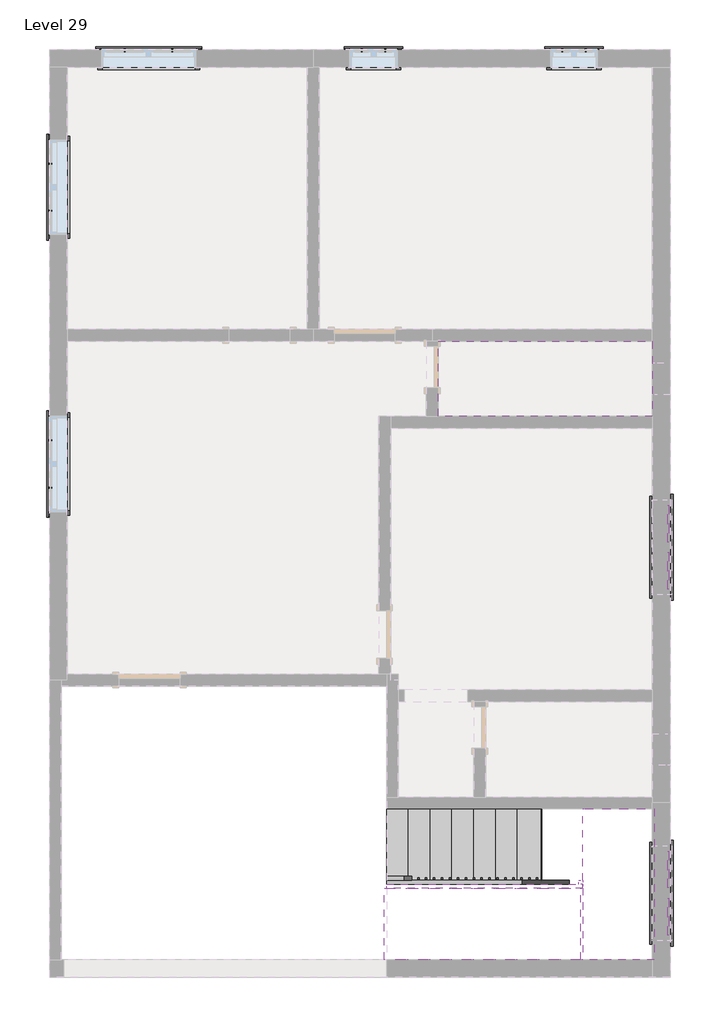
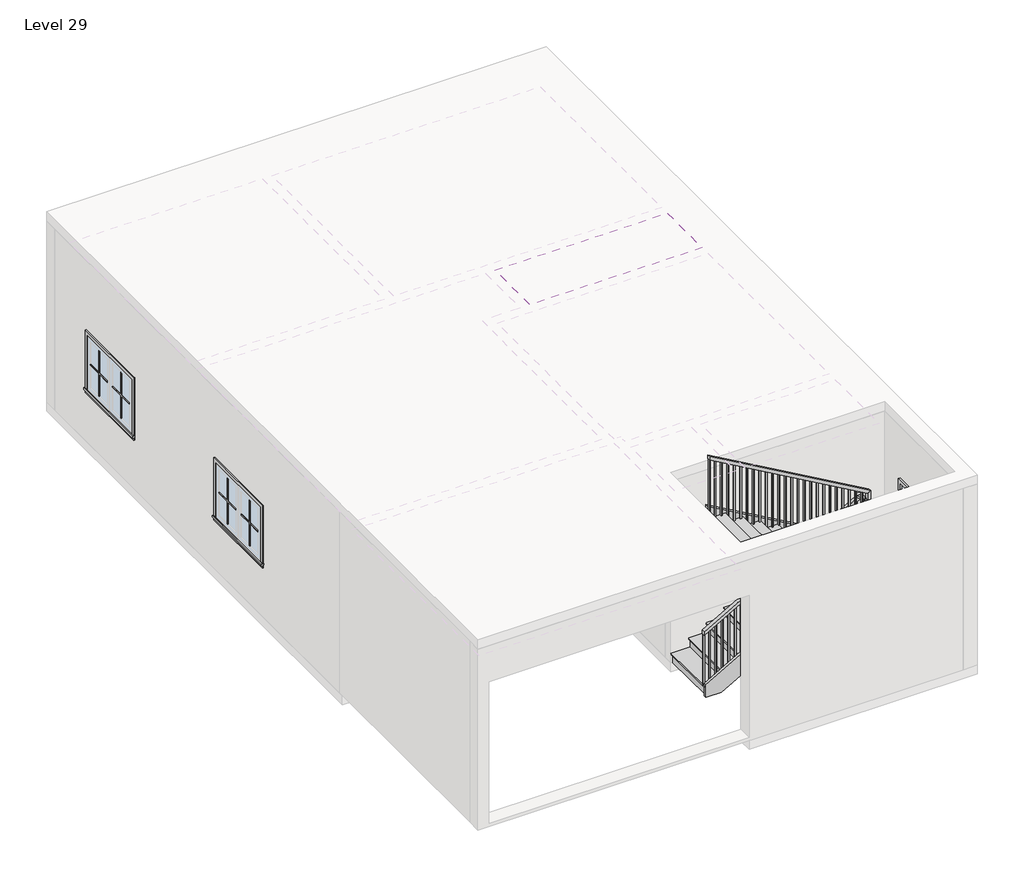
# One storey, part 2 of 2: 44 proxies, 3 members, 2 stair flights, 1 covering, 1 railing, 1 slab.
"""IFC4 building model written with IfcOpenShell, lengths in millimetres."""

from ifc_helpers import new_model, si_unit, frame, origin, place, context, project, spatial, polyline, outline, extrude, faceted_brep, transform, mapped, element, save
from components import muntin_pattern_2x2_muntin_pattern_2x2_2357e71d, muntin_pattern_2x2_muntin_pattern_2x2_302d8f29, muntin_pattern_2x2_muntin_pattern_2x2_53152e2c, muntin_pattern_2x2_muntin_pattern_2x2_e8f3e573, trim_window_exterior_flat_with_sill_c4e67c73, trim_window_exterior_flat_with_sill_a665a915, trim_window_interior_flat_picture_frame_cf1733af, trim_window_interior_flat_picture_frame_d485c387, non_monolithic_landing_9a06da9a, stair_flight_ff2ce9cd, stair_flight_de0ef723

model = new_model("IFC4")

# Units and contexts
model_context = context("Model", 3, world=origin())
ifc_project = project(units=[si_unit("LENGTHUNIT", "METRE", prefix="MILLI")], contexts=[model_context])

# Site, building, storey
site = spatial("IfcSite", under=ifc_project)
building = spatial("IfcBuilding", under=site)
storey = spatial("IfcBuildingStorey", under=building, Name="Level 29", Elevation=25603.2)

# Proxies
placement = place(None, origin())
muntin_pattern_2x2_muntin_pattern_2x2_shape = muntin_pattern_2x2_muntin_pattern_2x2_2357e71d(model_context)
element("IfcBuildingElementProxy", 1, Name="Muntin Pattern_2x2 : Muntin Pattern_2x2", ObjectType="Muntin Pattern_2x2 : Muntin Pattern_2x2", at=placement, inside=storey, context=model_context, shape_type="MappedRepresentation", body=[
    mapped(muntin_pattern_2x2_muntin_pattern_2x2_shape, transform((-4942.3279463, 5897.3080275, 26587.45), x_axis=(1.0, 0.0, 0.0), y_axis=(0.0, 1.0, 0.0), z_axis=(0.0, 0.0, 1.0))),
])
element("IfcBuildingElementProxy", 2, Name="Muntin Pattern_2x2 : Muntin Pattern_2x2", ObjectType="Muntin Pattern_2x2 : Muntin Pattern_2x2", at=placement, inside=storey, context=model_context, shape_type="MappedRepresentation", body=[
    mapped(muntin_pattern_2x2_muntin_pattern_2x2_shape, transform((-5899.5904463, 3838.3205275, 26587.45), x_axis=(0.0, 1.0, 0.0), y_axis=(-1.0, 0.0, 0.0), z_axis=(0.0, 0.0, 1.0))),
])
element("IfcBuildingElementProxy", 3, Name="Muntin Pattern_2x2 : Muntin Pattern_2x2", ObjectType="Muntin Pattern_2x2 : Muntin Pattern_2x2", at=placement, inside=storey, context=model_context, shape_type="MappedRepresentation", body=[
    mapped(muntin_pattern_2x2_muntin_pattern_2x2_shape, transform((-5899.5904463, 293.4330275, 26587.45), x_axis=(0.0, 1.0, 0.0), y_axis=(-1.0, 0.0, 0.0), z_axis=(0.0, 0.0, 1.0))),
])
element("IfcBuildingElementProxy", 4, Name="Muntin Pattern_2x2 : Muntin Pattern_2x2", ObjectType="Muntin Pattern_2x2 : Muntin Pattern_2x2", at=placement, inside=storey, context=model_context, shape_type="MappedRepresentation", body=[
    mapped(muntin_pattern_2x2_muntin_pattern_2x2_shape, transform((2031.5595537, -166.9419725, 26892.25), x_axis=(0.0, -1.0, 0.0), y_axis=(1.0, 0.0, 0.0), z_axis=(0.0, 0.0, 1.0))),
])
element("IfcBuildingElementProxy", 5, Name="Muntin Pattern_2x2 : Muntin Pattern_2x2", ObjectType="Muntin Pattern_2x2 : Muntin Pattern_2x2", at=placement, inside=storey, context=model_context, shape_type="MappedRepresentation", body=[
    mapped(muntin_pattern_2x2_muntin_pattern_2x2_shape, transform((2031.5595537, -4599.2419725, 26892.25), x_axis=(0.0, -1.0, 0.0), y_axis=(1.0, 0.0, 0.0), z_axis=(0.0, 0.0, 1.0))),
])
element("IfcBuildingElementProxy", 6, Name="Muntin Pattern_2x2 : Muntin Pattern_2x2", ObjectType="Muntin Pattern_2x2 : Muntin Pattern_2x2", at=placement, inside=storey, context=model_context, shape_type="MappedRepresentation", body=[
    mapped(muntin_pattern_2x2_muntin_pattern_2x2_shape, transform((-4942.3279463, 5897.3080275, 26587.45), x_axis=(1.0, 0.0, 0.0), y_axis=(0.0, 1.0, 0.0), z_axis=(0.0, 0.0, 1.0))),
])
element("IfcBuildingElementProxy", 7, Name="Muntin Pattern_2x2 : Muntin Pattern_2x2", ObjectType="Muntin Pattern_2x2 : Muntin Pattern_2x2", at=placement, inside=storey, context=model_context, shape_type="MappedRepresentation", body=[
    mapped(muntin_pattern_2x2_muntin_pattern_2x2_shape, transform((2031.5595537, -4599.2419725, 26892.25), x_axis=(0.0, -1.0, 0.0), y_axis=(1.0, 0.0, 0.0), z_axis=(0.0, 0.0, 1.0))),
])
muntin_pattern_2x2_muntin_pattern_2x2_2_shape = muntin_pattern_2x2_muntin_pattern_2x2_302d8f29(model_context)
element("IfcBuildingElementProxy", 8, Name="Muntin Pattern_2x2 : Muntin Pattern_2x2", ObjectType="Muntin Pattern_2x2 : Muntin Pattern_2x2", at=placement, inside=storey, context=model_context, shape_type="MappedRepresentation", body=[
    mapped(muntin_pattern_2x2_muntin_pattern_2x2_2_shape, transform((-4335.9029463, 5897.3080275, 26587.45), x_axis=(-1.0, 0.0, 0.0), y_axis=(0.0, -1.0, 0.0), z_axis=(0.0, 0.0, 1.0))),
])
element("IfcBuildingElementProxy", 9, Name="Muntin Pattern_2x2 : Muntin Pattern_2x2", ObjectType="Muntin Pattern_2x2 : Muntin Pattern_2x2", at=placement, inside=storey, context=model_context, shape_type="MappedRepresentation", body=[
    mapped(muntin_pattern_2x2_muntin_pattern_2x2_2_shape, transform((-5899.5904463, 4444.7455275, 26587.45), x_axis=(0.0, -1.0, 0.0), y_axis=(1.0, 0.0, 0.0), z_axis=(0.0, 0.0, 1.0))),
])
element("IfcBuildingElementProxy", 10, Name="Muntin Pattern_2x2 : Muntin Pattern_2x2", ObjectType="Muntin Pattern_2x2 : Muntin Pattern_2x2", at=placement, inside=storey, context=model_context, shape_type="MappedRepresentation", body=[
    mapped(muntin_pattern_2x2_muntin_pattern_2x2_2_shape, transform((-5899.5904463, 899.8580275, 26587.45), x_axis=(0.0, -1.0, 0.0), y_axis=(1.0, 0.0, 0.0), z_axis=(0.0, 0.0, 1.0))),
])
element("IfcBuildingElementProxy", 11, Name="Muntin Pattern_2x2 : Muntin Pattern_2x2", ObjectType="Muntin Pattern_2x2 : Muntin Pattern_2x2", at=placement, inside=storey, context=model_context, shape_type="MappedRepresentation", body=[
    mapped(muntin_pattern_2x2_muntin_pattern_2x2_2_shape, transform((2031.5595537, -773.3669725, 26892.25), x_axis=(0.0, 1.0, 0.0), y_axis=(-1.0, 0.0, 0.0), z_axis=(0.0, 0.0, 1.0))),
])
element("IfcBuildingElementProxy", 12, Name="Muntin Pattern_2x2 : Muntin Pattern_2x2", ObjectType="Muntin Pattern_2x2 : Muntin Pattern_2x2", at=placement, inside=storey, context=model_context, shape_type="MappedRepresentation", body=[
    mapped(muntin_pattern_2x2_muntin_pattern_2x2_2_shape, transform((2031.5595537, -5205.6669725, 26892.25), x_axis=(0.0, 1.0, 0.0), y_axis=(-1.0, 0.0, 0.0), z_axis=(0.0, 0.0, 1.0))),
])
element("IfcBuildingElementProxy", 13, Name="Muntin Pattern_2x2 : Muntin Pattern_2x2", ObjectType="Muntin Pattern_2x2 : Muntin Pattern_2x2", at=placement, inside=storey, context=model_context, shape_type="MappedRepresentation", body=[
    mapped(muntin_pattern_2x2_muntin_pattern_2x2_2_shape, transform((-4335.9029463, 5897.3080275, 26587.45), x_axis=(-1.0, 0.0, 0.0), y_axis=(0.0, -1.0, 0.0), z_axis=(0.0, 0.0, 1.0))),
])
element("IfcBuildingElementProxy", 14, Name="Muntin Pattern_2x2 : Muntin Pattern_2x2", ObjectType="Muntin Pattern_2x2 : Muntin Pattern_2x2", at=placement, inside=storey, context=model_context, shape_type="MappedRepresentation", body=[
    mapped(muntin_pattern_2x2_muntin_pattern_2x2_2_shape, transform((2031.5595537, -5205.6669725, 26892.25), x_axis=(0.0, 1.0, 0.0), y_axis=(-1.0, 0.0, 0.0), z_axis=(0.0, 0.0, 1.0))),
])
muntin_pattern_2x2_muntin_pattern_2x2_3_shape = muntin_pattern_2x2_muntin_pattern_2x2_53152e2c(model_context)
element("IfcBuildingElementProxy", 15, Name="Muntin Pattern_2x2 : Muntin Pattern_2x2", ObjectType="Muntin Pattern_2x2 : Muntin Pattern_2x2", at=placement, inside=storey, context=model_context, shape_type="MappedRepresentation", body=[
    mapped(muntin_pattern_2x2_muntin_pattern_2x2_3_shape, transform((-1907.0279463, 5897.3080275, 26587.45), x_axis=(1.0, 0.0, 0.0), y_axis=(0.0, 1.0, 0.0), z_axis=(0.0, 0.0, 1.0))),
])
element("IfcBuildingElementProxy", 16, Name="Muntin Pattern_2x2 : Muntin Pattern_2x2", ObjectType="Muntin Pattern_2x2 : Muntin Pattern_2x2", at=placement, inside=storey, context=model_context, shape_type="MappedRepresentation", body=[
    mapped(muntin_pattern_2x2_muntin_pattern_2x2_3_shape, transform((658.3720537, 5897.3080275, 26587.45), x_axis=(1.0, 0.0, 0.0), y_axis=(0.0, 1.0, 0.0), z_axis=(0.0, 0.0, 1.0))),
])
element("IfcBuildingElementProxy", 17, Name="Muntin Pattern_2x2 : Muntin Pattern_2x2", ObjectType="Muntin Pattern_2x2 : Muntin Pattern_2x2", at=placement, inside=storey, context=model_context, shape_type="MappedRepresentation", body=[
    mapped(muntin_pattern_2x2_muntin_pattern_2x2_3_shape, transform((-1907.0279463, 5897.3080275, 26587.45), x_axis=(1.0, 0.0, 0.0), y_axis=(0.0, 1.0, 0.0), z_axis=(0.0, 0.0, 1.0))),
])
element("IfcBuildingElementProxy", 18, Name="Muntin Pattern_2x2 : Muntin Pattern_2x2", ObjectType="Muntin Pattern_2x2 : Muntin Pattern_2x2", at=placement, inside=storey, context=model_context, shape_type="MappedRepresentation", body=[
    mapped(muntin_pattern_2x2_muntin_pattern_2x2_3_shape, transform((658.3720537, 5897.3080275, 26587.45), x_axis=(1.0, 0.0, 0.0), y_axis=(0.0, 1.0, 0.0), z_axis=(0.0, 0.0, 1.0))),
])
muntin_pattern_2x2_muntin_pattern_2x2_4_shape = muntin_pattern_2x2_muntin_pattern_2x2_e8f3e573(model_context)
element("IfcBuildingElementProxy", 19, Name="Muntin Pattern_2x2 : Muntin Pattern_2x2", ObjectType="Muntin Pattern_2x2 : Muntin Pattern_2x2", at=placement, inside=storey, context=model_context, shape_type="MappedRepresentation", body=[
    mapped(muntin_pattern_2x2_muntin_pattern_2x2_4_shape, transform((-1605.4029463, 5897.3080275, 26587.45), x_axis=(-1.0, 0.0, 0.0), y_axis=(0.0, -1.0, 0.0), z_axis=(0.0, 0.0, 1.0))),
])
element("IfcBuildingElementProxy", 20, Name="Muntin Pattern_2x2 : Muntin Pattern_2x2", ObjectType="Muntin Pattern_2x2 : Muntin Pattern_2x2", at=placement, inside=storey, context=model_context, shape_type="MappedRepresentation", body=[
    mapped(muntin_pattern_2x2_muntin_pattern_2x2_4_shape, transform((959.9970537, 5897.3080275, 26587.45), x_axis=(-1.0, 0.0, 0.0), y_axis=(0.0, -1.0, 0.0), z_axis=(0.0, 0.0, 1.0))),
])
element("IfcBuildingElementProxy", 21, Name="Muntin Pattern_2x2 : Muntin Pattern_2x2", ObjectType="Muntin Pattern_2x2 : Muntin Pattern_2x2", at=placement, inside=storey, context=model_context, shape_type="MappedRepresentation", body=[
    mapped(muntin_pattern_2x2_muntin_pattern_2x2_4_shape, transform((-1605.4029463, 5897.3080275, 26587.45), x_axis=(-1.0, 0.0, 0.0), y_axis=(0.0, -1.0, 0.0), z_axis=(0.0, 0.0, 1.0))),
])
element("IfcBuildingElementProxy", 22, Name="Muntin Pattern_2x2 : Muntin Pattern_2x2", ObjectType="Muntin Pattern_2x2 : Muntin Pattern_2x2", at=placement, inside=storey, context=model_context, shape_type="MappedRepresentation", body=[
    mapped(muntin_pattern_2x2_muntin_pattern_2x2_4_shape, transform((959.9970537, 5897.3080275, 26587.45), x_axis=(-1.0, 0.0, 0.0), y_axis=(0.0, -1.0, 0.0), z_axis=(0.0, 0.0, 1.0))),
])
trim_window_exterior_flat_with_sill_shape = trim_window_exterior_flat_with_sill_c4e67c73(model_context)
element("IfcBuildingElementProxy", 23, Name="Trim-Window-Exterior-Flat : with Sill", ObjectType="Trim-Window-Exterior-Flat : with Sill", at=placement, inside=storey, context=model_context, shape_type="MappedRepresentation", body=[
    mapped(trim_window_exterior_flat_with_sill_shape, transform((-4639.1154463, 5906.8330275, 27432.0), x_axis=(-1.0, 0.0, 0.0), y_axis=(0.0, 0.0, 1.0), z_axis=(0.0, 1.0, 0.0))),
])
element("IfcBuildingElementProxy", 24, Name="Trim-Window-Exterior-Flat : with Sill", ObjectType="Trim-Window-Exterior-Flat : with Sill", at=placement, inside=storey, context=model_context, shape_type="MappedRepresentation", body=[
    mapped(trim_window_exterior_flat_with_sill_shape, transform((-5909.1154463, 4141.5330275, 27432.0), x_axis=(0.0, -1.0, 0.0), y_axis=(0.0, 0.0, 1.0), z_axis=(-1.0, 0.0, 0.0))),
])
element("IfcBuildingElementProxy", 25, Name="Trim-Window-Exterior-Flat : with Sill", ObjectType="Trim-Window-Exterior-Flat : with Sill", at=placement, inside=storey, context=model_context, shape_type="MappedRepresentation", body=[
    mapped(trim_window_exterior_flat_with_sill_shape, transform((-5909.1154463, 596.6455275, 27432.0), x_axis=(0.0, -1.0, 0.0), y_axis=(0.0, 0.0, 1.0), z_axis=(-1.0, 0.0, 0.0))),
])
element("IfcBuildingElementProxy", 26, Name="Trim-Window-Exterior-Flat : with Sill", ObjectType="Trim-Window-Exterior-Flat : with Sill", at=placement, inside=storey, context=model_context, shape_type="MappedRepresentation", body=[
    mapped(trim_window_exterior_flat_with_sill_shape, transform((2041.0845537, -470.1544725, 27736.8), x_axis=(0.0, 1.0, 0.0), y_axis=(0.0, 0.0, 1.0), z_axis=(1.0, 0.0, 0.0))),
])
element("IfcBuildingElementProxy", 27, Name="Trim-Window-Exterior-Flat : with Sill", ObjectType="Trim-Window-Exterior-Flat : with Sill", at=placement, inside=storey, context=model_context, shape_type="MappedRepresentation", body=[
    mapped(trim_window_exterior_flat_with_sill_shape, transform((2041.0845537, -4902.4544725, 27736.8), x_axis=(0.0, 1.0, 0.0), y_axis=(0.0, 0.0, 1.0), z_axis=(1.0, 0.0, 0.0))),
])
element("IfcBuildingElementProxy", 28, Name="Trim-Window-Exterior-Flat : with Sill", ObjectType="Trim-Window-Exterior-Flat : with Sill", at=placement, inside=storey, context=model_context, shape_type="MappedRepresentation", body=[
    mapped(trim_window_exterior_flat_with_sill_shape, transform((-4639.1154463, 5906.8330275, 27432.0), x_axis=(-1.0, 0.0, 0.0), y_axis=(0.0, 0.0, 1.0), z_axis=(0.0, 1.0, 0.0))),
])
element("IfcBuildingElementProxy", 29, Name="Trim-Window-Exterior-Flat : with Sill", ObjectType="Trim-Window-Exterior-Flat : with Sill", at=placement, inside=storey, context=model_context, shape_type="MappedRepresentation", body=[
    mapped(trim_window_exterior_flat_with_sill_shape, transform((2041.0845537, -4902.4544725, 27736.8), x_axis=(0.0, 1.0, 0.0), y_axis=(0.0, 0.0, 1.0), z_axis=(1.0, 0.0, 0.0))),
])
trim_window_exterior_flat_with_sill_2_shape = trim_window_exterior_flat_with_sill_a665a915(model_context)
element("IfcBuildingElementProxy", 30, Name="Trim-Window-Exterior-Flat : with Sill", ObjectType="Trim-Window-Exterior-Flat : with Sill", at=placement, inside=storey, context=model_context, shape_type="MappedRepresentation", body=[
    mapped(trim_window_exterior_flat_with_sill_2_shape, transform((-1756.2154463, 5906.8330275, 27432.0), x_axis=(-1.0, 0.0, 0.0), y_axis=(0.0, 0.0, 1.0), z_axis=(0.0, 1.0, 0.0))),
])
element("IfcBuildingElementProxy", 31, Name="Trim-Window-Exterior-Flat : with Sill", ObjectType="Trim-Window-Exterior-Flat : with Sill", at=placement, inside=storey, context=model_context, shape_type="MappedRepresentation", body=[
    mapped(trim_window_exterior_flat_with_sill_2_shape, transform((809.1845537, 5906.8330275, 27432.0), x_axis=(-1.0, 0.0, 0.0), y_axis=(0.0, 0.0, 1.0), z_axis=(0.0, 1.0, 0.0))),
])
element("IfcBuildingElementProxy", 32, Name="Trim-Window-Exterior-Flat : with Sill", ObjectType="Trim-Window-Exterior-Flat : with Sill", at=placement, inside=storey, context=model_context, shape_type="MappedRepresentation", body=[
    mapped(trim_window_exterior_flat_with_sill_2_shape, transform((-1756.2154463, 5906.8330275, 27432.0), x_axis=(-1.0, 0.0, 0.0), y_axis=(0.0, 0.0, 1.0), z_axis=(0.0, 1.0, 0.0))),
])
element("IfcBuildingElementProxy", 33, Name="Trim-Window-Exterior-Flat : with Sill", ObjectType="Trim-Window-Exterior-Flat : with Sill", at=placement, inside=storey, context=model_context, shape_type="MappedRepresentation", body=[
    mapped(trim_window_exterior_flat_with_sill_2_shape, transform((809.1845537, 5906.8330275, 27432.0), x_axis=(-1.0, 0.0, 0.0), y_axis=(0.0, 0.0, 1.0), z_axis=(0.0, 1.0, 0.0))),
])
trim_window_interior_flat_picture_frame_shape = trim_window_interior_flat_picture_frame_cf1733af(model_context)
element("IfcBuildingElementProxy", 34, Name="Trim-Window-Interior-Flat : Picture Frame", ObjectType="Trim-Window-Interior-Flat : Picture Frame", at=placement, inside=storey, context=model_context, shape_type="MappedRepresentation", body=[
    mapped(trim_window_interior_flat_picture_frame_shape, transform((-4639.1154463, 5678.2330275, 27432.0), x_axis=(1.0, 0.0, 0.0), y_axis=(0.0, 0.0, 1.0), z_axis=(0.0, -1.0, 0.0))),
])
element("IfcBuildingElementProxy", 35, Name="Trim-Window-Interior-Flat : Picture Frame", ObjectType="Trim-Window-Interior-Flat : Picture Frame", at=placement, inside=storey, context=model_context, shape_type="MappedRepresentation", body=[
    mapped(trim_window_interior_flat_picture_frame_shape, transform((-5680.5154463, 4141.5330275, 27432.0), x_axis=(0.0, 1.0, 0.0), y_axis=(0.0, 0.0, 1.0), z_axis=(1.0, 0.0, 0.0))),
])
element("IfcBuildingElementProxy", 36, Name="Trim-Window-Interior-Flat : Picture Frame", ObjectType="Trim-Window-Interior-Flat : Picture Frame", at=placement, inside=storey, context=model_context, shape_type="MappedRepresentation", body=[
    mapped(trim_window_interior_flat_picture_frame_shape, transform((-5680.5154463, 596.6455275, 27432.0), x_axis=(0.0, 1.0, 0.0), y_axis=(0.0, 0.0, 1.0), z_axis=(1.0, 0.0, 0.0))),
])
element("IfcBuildingElementProxy", 37, Name="Trim-Window-Interior-Flat : Picture Frame", ObjectType="Trim-Window-Interior-Flat : Picture Frame", at=placement, inside=storey, context=model_context, shape_type="MappedRepresentation", body=[
    mapped(trim_window_interior_flat_picture_frame_shape, transform((1812.4845537, -470.1544725, 27736.8), x_axis=(0.0, -1.0, 0.0), y_axis=(0.0, 0.0, 1.0), z_axis=(-1.0, 0.0, 0.0))),
])
element("IfcBuildingElementProxy", 38, Name="Trim-Window-Interior-Flat : Picture Frame", ObjectType="Trim-Window-Interior-Flat : Picture Frame", at=placement, inside=storey, context=model_context, shape_type="MappedRepresentation", body=[
    mapped(trim_window_interior_flat_picture_frame_shape, transform((1812.4845537, -4902.4544725, 27736.8), x_axis=(0.0, -1.0, 0.0), y_axis=(0.0, 0.0, 1.0), z_axis=(-1.0, 0.0, 0.0))),
])
element("IfcBuildingElementProxy", 39, Name="Trim-Window-Interior-Flat : Picture Frame", ObjectType="Trim-Window-Interior-Flat : Picture Frame", at=placement, inside=storey, context=model_context, shape_type="MappedRepresentation", body=[
    mapped(trim_window_interior_flat_picture_frame_shape, transform((-4639.1154463, 5678.2330275, 27432.0), x_axis=(1.0, 0.0, 0.0), y_axis=(0.0, 0.0, 1.0), z_axis=(0.0, -1.0, 0.0))),
])
element("IfcBuildingElementProxy", 40, Name="Trim-Window-Interior-Flat : Picture Frame", ObjectType="Trim-Window-Interior-Flat : Picture Frame", at=placement, inside=storey, context=model_context, shape_type="MappedRepresentation", body=[
    mapped(trim_window_interior_flat_picture_frame_shape, transform((1812.4845537, -4902.4544725, 27736.8), x_axis=(0.0, -1.0, 0.0), y_axis=(0.0, 0.0, 1.0), z_axis=(-1.0, 0.0, 0.0))),
])
trim_window_interior_flat_picture_frame_2_shape = trim_window_interior_flat_picture_frame_d485c387(model_context)
element("IfcBuildingElementProxy", 41, Name="Trim-Window-Interior-Flat : Picture Frame", ObjectType="Trim-Window-Interior-Flat : Picture Frame", at=placement, inside=storey, context=model_context, shape_type="MappedRepresentation", body=[
    mapped(trim_window_interior_flat_picture_frame_2_shape, transform((-1756.2154463, 5678.2330275, 27432.0), x_axis=(1.0, 0.0, 0.0), y_axis=(0.0, 0.0, 1.0), z_axis=(0.0, -1.0, 0.0))),
])
element("IfcBuildingElementProxy", 42, Name="Trim-Window-Interior-Flat : Picture Frame", ObjectType="Trim-Window-Interior-Flat : Picture Frame", at=placement, inside=storey, context=model_context, shape_type="MappedRepresentation", body=[
    mapped(trim_window_interior_flat_picture_frame_2_shape, transform((809.1845537, 5678.2330275, 27432.0), x_axis=(1.0, 0.0, 0.0), y_axis=(0.0, 0.0, 1.0), z_axis=(0.0, -1.0, 0.0))),
])
element("IfcBuildingElementProxy", 43, Name="Trim-Window-Interior-Flat : Picture Frame", ObjectType="Trim-Window-Interior-Flat : Picture Frame", at=placement, inside=storey, context=model_context, shape_type="MappedRepresentation", body=[
    mapped(trim_window_interior_flat_picture_frame_2_shape, transform((-1756.2154463, 5678.2330275, 27432.0), x_axis=(1.0, 0.0, 0.0), y_axis=(0.0, 0.0, 1.0), z_axis=(0.0, -1.0, 0.0))),
])
element("IfcBuildingElementProxy", 44, Name="Trim-Window-Interior-Flat : Picture Frame", ObjectType="Trim-Window-Interior-Flat : Picture Frame", at=placement, inside=storey, context=model_context, shape_type="MappedRepresentation", body=[
    mapped(trim_window_interior_flat_picture_frame_2_shape, transform((809.1845537, 5678.2330275, 27432.0), x_axis=(1.0, 0.0, 0.0), y_axis=(0.0, 0.0, 1.0), z_axis=(0.0, -1.0, 0.0))),
])

# Covering
element("IfcCovering", 45, ObjectType="2' x 4' ACT System", at=placement, inside=storey, context=model_context, shape_type="SweptSolid", body=[
    extrude(outline(polyline([(-930.7154463, 2171.4455275), (1812.4845537, 2171.4455275), (1812.4845537, 1206.2455275), (-930.7154463, 1206.2455275), (-930.7154463, 2171.4455275)])), frame((0.0, 0.0, 28346.4), z_axis=(0.0, 0.0, 1.0), x_axis=(1.0, 0.0, 0.0)), (0.0, 0.0, 1.0), 57.15),
])

# Members
element("IfcMember", 46, ObjectType="Stringer - 2\" Width", at=placement, inside=storey, context=model_context, shape_type="SweptSolid", body=[
    extrude(outline(polyline([(25812.2890626, -1591.1154463), (25603.2, -1591.1154463), (25603.2, -1342.8974141), (26872.124218, 872.6845537), (27223.3745172, 872.6845537), (25812.2890626, -1591.1154463)])), frame((0.0, -4788.1544725, 0.0), z_axis=(0.0, 1.0, 0.0), x_axis=(0.0, 0.0, 1.0)), (0.0, 0.0, 1.0), 50.8),
])
element("IfcMember", 47, ObjectType="Stringer - 2\" Width", at=placement, inside=storey, context=model_context, shape_type="SweptSolid", body=[
    extrude(outline(polyline([(27061.2387634, 923.4845537), (27412.4890626, 923.4845537), (28852.6690626, -1591.1154463), (28501.4187634, -1591.1154463), (27061.2387634, 923.4845537)])), frame((0.0, -4838.9544725, 0.0), z_axis=(0.0, 1.0, 0.0), x_axis=(0.0, 0.0, 1.0)), (0.0, 0.0, 1.0), 50.8),
])
element("IfcMember", 48, ObjectType="Stringer - 2\" Width", at=placement, inside=storey, context=model_context, shape_type="SweptSolid", body=[
    extrude(outline(polyline([(872.6845537, -4737.3544725), (923.4845537, -4737.3544725), (923.4845537, -4788.1544725), (872.6845537, -4788.1544725), (872.6845537, -4737.3544725)])), frame((0.0, 0.0, 26974.8), z_axis=(0.0, 0.0, 1.0), x_axis=(1.0, 0.0, 0.0)), (0.0, 0.0, 1.0), 304.8),
])

# Railing
element("IfcRailing", 49, ObjectType="Handrail - Rectangular", at=placement, inside=storey, context=model_context, shape_type="SolidModel", body=[
    faceted_brep([(-1591.1154463, -4686.5544725, 26677.62), (-1591.1154463, -4686.5544725, 26619.0782835), (-1591.1154463, -4737.3544725, 26619.0782835), (-1591.1154463, -4737.3544725, 26677.62), (847.2845537, -4686.5544725, 28074.1581818), (898.0845537, -4686.5544725, 28044.7110107), (898.0845537, -4737.3544725, 28044.7110107), (847.2845537, -4737.3544725, 28074.1581818), (847.2845537, -4686.5544725, 28117.8), (898.0845537, -4686.5544725, 28067.0), (898.0845537, -4737.3544725, 28067.0), (847.2845537, -4737.3544725, 28117.8), (974.2845537, -4686.5544725, 28117.8), (974.2845537, -4686.5544725, 28067.0), (923.4845537, -4737.3544725, 28067.0), (923.4845537, -4737.3544725, 28117.8), (974.2845537, -4813.5544725, 28117.8), (974.2845537, -4813.5544725, 28067.0), (923.4845537, -4813.5544725, 28067.0), (923.4845537, -4813.5544725, 28117.8), (974.2845537, -4838.9544725, 28117.8), (923.4845537, -4838.9544725, 28117.8), (923.4845537, -4889.7544725, 28067.0), (974.2845537, -4889.7544725, 28067.0)], [[[0, 1, 2, 3]], [[1, 0, 4, 5]], [[2, 1, 5, 6]], [[3, 2, 6, 7]], [[0, 3, 7, 4]], [[5, 4, 8, 9]], [[6, 5, 9, 10]], [[7, 6, 10, 11]], [[4, 7, 11, 8]], [[9, 8, 12, 13]], [[10, 9, 13, 14]], [[11, 10, 14, 15]], [[8, 11, 15, 12]], [[13, 12, 16, 17]], [[14, 13, 17, 18]], [[15, 14, 18, 19]], [[12, 15, 19, 16]], [[20, 21, 22, 23]], [[17, 16, 20, 23]], [[18, 17, 23, 22]], [[19, 18, 22, 21]], [[16, 19, 21, 20]]]),
    faceted_brep([(974.2845537, -4838.9544725, 28117.8), (974.2845537, -4889.7544725, 28067.0), (923.4845537, -4889.7544725, 28067.0), (923.4845537, -4838.9544725, 28117.8), (974.2845537, -4838.9544725, 28248.7254545), (923.4845537, -4838.9544725, 28219.2782835), (923.4845537, -4889.7544725, 28219.2782835), (974.2845537, -4889.7544725, 28248.7254545)], [[[0, 1, 2, 3]], [[4, 5, 6, 7]], [[1, 0, 4, 7]], [[2, 1, 7, 6]], [[3, 2, 6, 5]], [[0, 3, 5, 4]]]),
    faceted_brep([(974.2845537, -4889.7544725, 28248.7254545), (923.4845537, -4889.7544725, 28219.2782835), (923.4845537, -4838.9544725, 28219.2782835), (974.2845537, -4838.9544725, 28248.7254545), (-1591.1154463, -4889.7544725, 29718.0), (-1591.1154463, -4838.9544725, 29718.0), (-1591.1154463, -4838.9544725, 29659.4582835), (-1591.1154463, -4889.7544725, 29659.4582835)], [[[0, 1, 2, 3]], [[4, 5, 6, 7]], [[1, 0, 4, 7]], [[2, 1, 7, 6]], [[3, 2, 6, 5]], [[0, 3, 5, 4]]]),
    extrude(outline(polyline([(29595.8139653, -1479.9904463), (29606.7244198, -1499.0404463), (28643.58, -1499.0404463), (28643.58, -1479.9904463), (29595.8139653, -1479.9904463)])), frame((0.0, -4873.8794725, 0.0), z_axis=(0.0, 1.0, 0.0), x_axis=(0.0, 0.0, 1.0)), (0.0, 0.0, 1.0), 19.05),
    extrude(outline(polyline([(29537.6248744, -1378.3904463), (29548.5353289, -1397.4404463), (28643.58, -1397.4404463), (28643.58, -1378.3904463), (29537.6248744, -1378.3904463)])), frame((0.0, -4873.8794725, 0.0), z_axis=(0.0, 1.0, 0.0), x_axis=(0.0, 0.0, 1.0)), (0.0, 0.0, 1.0), 19.05),
    extrude(outline(polyline([(29479.4357835, -1276.7904463), (29490.346238, -1295.8404463), (28483.56, -1295.8404463), (28483.56, -1276.7904463), (29479.4357835, -1276.7904463)])), frame((0.0, -4873.8794725, 0.0), z_axis=(0.0, 1.0, 0.0), x_axis=(0.0, 0.0, 1.0)), (0.0, 0.0, 1.0), 19.05),
    extrude(outline(polyline([(29421.2466926, -1175.1904463), (29432.1571471, -1194.2404463), (28483.56, -1194.2404463), (28483.56, -1175.1904463), (29421.2466926, -1175.1904463)])), frame((0.0, -4873.8794725, 0.0), z_axis=(0.0, 1.0, 0.0), x_axis=(0.0, 0.0, 1.0)), (0.0, 0.0, 1.0), 19.05),
    extrude(outline(polyline([(29363.0576016, -1073.5904463), (29373.9680562, -1092.6404463), (28483.56, -1092.6404463), (28483.56, -1073.5904463), (29363.0576016, -1073.5904463)])), frame((0.0, -4873.8794725, 0.0), z_axis=(0.0, 1.0, 0.0), x_axis=(0.0, 0.0, 1.0)), (0.0, 0.0, 1.0), 19.05),
    extrude(outline(polyline([(29304.8685107, -971.9904463), (29315.7789653, -991.0404463), (28323.54, -991.0404463), (28323.54, -971.9904463), (29304.8685107, -971.9904463)])), frame((0.0, -4873.8794725, 0.0), z_axis=(0.0, 1.0, 0.0), x_axis=(0.0, 0.0, 1.0)), (0.0, 0.0, 1.0), 19.05),
    extrude(outline(polyline([(29246.6794198, -870.3904463), (29257.5898744, -889.4404463), (28323.54, -889.4404463), (28323.54, -870.3904463), (29246.6794198, -870.3904463)])), frame((0.0, -4873.8794725, 0.0), z_axis=(0.0, 1.0, 0.0), x_axis=(0.0, 0.0, 1.0)), (0.0, 0.0, 1.0), 19.05),
    extrude(outline(polyline([(29188.4903289, -768.7904463), (29199.4007835, -787.8404463), (28323.54, -787.8404463), (28323.54, -768.7904463), (29188.4903289, -768.7904463)])), frame((0.0, -4873.8794725, 0.0), z_axis=(0.0, 1.0, 0.0), x_axis=(0.0, 0.0, 1.0)), (0.0, 0.0, 1.0), 19.05),
    extrude(outline(polyline([(29130.301238, -667.1904463), (29141.2116926, -686.2404463), (28163.52, -686.2404463), (28163.52, -667.1904463), (29130.301238, -667.1904463)])), frame((0.0, -4873.8794725, 0.0), z_axis=(0.0, 1.0, 0.0), x_axis=(0.0, 0.0, 1.0)), (0.0, 0.0, 1.0), 19.05),
    extrude(outline(polyline([(29072.1121471, -565.5904463), (29083.0226016, -584.6404463), (28163.52, -584.6404463), (28163.52, -565.5904463), (29072.1121471, -565.5904463)])), frame((0.0, -4873.8794725, 0.0), z_axis=(0.0, 1.0, 0.0), x_axis=(0.0, 0.0, 1.0)), (0.0, 0.0, 1.0), 19.05),
    extrude(outline(polyline([(29013.9230562, -463.9904463), (29024.8335107, -483.0404463), (28163.52, -483.0404463), (28163.52, -463.9904463), (29013.9230562, -463.9904463)])), frame((0.0, -4873.8794725, 0.0), z_axis=(0.0, 1.0, 0.0), x_axis=(0.0, 0.0, 1.0)), (0.0, 0.0, 1.0), 19.05),
    extrude(outline(polyline([(28955.7339653, -362.3904463), (28966.6444198, -381.4404463), (28003.5, -381.4404463), (28003.5, -362.3904463), (28955.7339653, -362.3904463)])), frame((0.0, -4873.8794725, 0.0), z_axis=(0.0, 1.0, 0.0), x_axis=(0.0, 0.0, 1.0)), (0.0, 0.0, 1.0), 19.05),
    extrude(outline(polyline([(28897.5448744, -260.7904463), (28908.4553289, -279.8404463), (28003.5, -279.8404463), (28003.5, -260.7904463), (28897.5448744, -260.7904463)])), frame((0.0, -4873.8794725, 0.0), z_axis=(0.0, 1.0, 0.0), x_axis=(0.0, 0.0, 1.0)), (0.0, 0.0, 1.0), 19.05),
    extrude(outline(polyline([(28839.3557835, -159.1904463), (28850.266238, -178.2404463), (27843.48, -178.2404463), (27843.48, -159.1904463), (28839.3557835, -159.1904463)])), frame((0.0, -4873.8794725, 0.0), z_axis=(0.0, 1.0, 0.0), x_axis=(0.0, 0.0, 1.0)), (0.0, 0.0, 1.0), 19.05),
    extrude(outline(polyline([(28781.1666926, -57.5904463), (28792.0771471, -76.6404463), (27843.48, -76.6404463), (27843.48, -57.5904463), (28781.1666926, -57.5904463)])), frame((0.0, -4873.8794725, 0.0), z_axis=(0.0, 1.0, 0.0), x_axis=(0.0, 0.0, 1.0)), (0.0, 0.0, 1.0), 19.05),
    extrude(outline(polyline([(28722.9776016, 44.0095537), (28733.8880562, 24.9595537), (27843.48, 24.9595537), (27843.48, 44.0095537), (28722.9776016, 44.0095537)])), frame((0.0, -4873.8794725, 0.0), z_axis=(0.0, 1.0, 0.0), x_axis=(0.0, 0.0, 1.0)), (0.0, 0.0, 1.0), 19.05),
    extrude(outline(polyline([(28664.7885107, 145.6095537), (28675.6989653, 126.5595537), (27683.46, 126.5595537), (27683.46, 145.6095537), (28664.7885107, 145.6095537)])), frame((0.0, -4873.8794725, 0.0), z_axis=(0.0, 1.0, 0.0), x_axis=(0.0, 0.0, 1.0)), (0.0, 0.0, 1.0), 19.05),
    extrude(outline(polyline([(28606.5994198, 247.2095537), (28617.5098744, 228.1595537), (27683.46, 228.1595537), (27683.46, 247.2095537), (28606.5994198, 247.2095537)])), frame((0.0, -4873.8794725, 0.0), z_axis=(0.0, 1.0, 0.0), x_axis=(0.0, 0.0, 1.0)), (0.0, 0.0, 1.0), 19.05),
    extrude(outline(polyline([(28548.4103289, 348.8095537), (28559.3207835, 329.7595537), (27683.46, 329.7595537), (27683.46, 348.8095537), (28548.4103289, 348.8095537)])), frame((0.0, -4873.8794725, 0.0), z_axis=(0.0, 1.0, 0.0), x_axis=(0.0, 0.0, 1.0)), (0.0, 0.0, 1.0), 19.05),
    extrude(outline(polyline([(28490.221238, 450.4095537), (28501.1316926, 431.3595537), (27523.44, 431.3595537), (27523.44, 450.4095537), (28490.221238, 450.4095537)])), frame((0.0, -4873.8794725, 0.0), z_axis=(0.0, 1.0, 0.0), x_axis=(0.0, 0.0, 1.0)), (0.0, 0.0, 1.0), 19.05),
    extrude(outline(polyline([(28432.0321471, 552.0095537), (28442.9426016, 532.9595537), (27523.44, 532.9595537), (27523.44, 552.0095537), (28432.0321471, 552.0095537)])), frame((0.0, -4873.8794725, 0.0), z_axis=(0.0, 1.0, 0.0), x_axis=(0.0, 0.0, 1.0)), (0.0, 0.0, 1.0), 19.05),
    extrude(outline(polyline([(28373.8430562, 653.6095537), (28384.7535107, 634.5595537), (27523.44, 634.5595537), (27523.44, 653.6095537), (28373.8430562, 653.6095537)])), frame((0.0, -4873.8794725, 0.0), z_axis=(0.0, 1.0, 0.0), x_axis=(0.0, 0.0, 1.0)), (0.0, 0.0, 1.0), 19.05),
    extrude(outline(polyline([(28315.6539653, 755.2095537), (28326.5644198, 736.1595537), (27363.42, 736.1595537), (27363.42, 755.2095537), (28315.6539653, 755.2095537)])), frame((0.0, -4873.8794725, 0.0), z_axis=(0.0, 1.0, 0.0), x_axis=(0.0, 0.0, 1.0)), (0.0, 0.0, 1.0), 19.05),
    extrude(outline(polyline([(28257.4648744, 856.8095537), (28268.3753289, 837.7595537), (27363.42, 837.7595537), (27363.42, 856.8095537), (28257.4648744, 856.8095537)])), frame((0.0, -4873.8794725, 0.0), z_axis=(0.0, 1.0, 0.0), x_axis=(0.0, 0.0, 1.0)), (0.0, 0.0, 1.0), 19.05),
    extrude(outline(polyline([(939.3595537, -4804.0294725), (958.4095537, -4804.0294725), (958.4095537, -4823.0794725), (939.3595537, -4823.0794725), (939.3595537, -4804.0294725)])), frame((0.0, 0.0, 27203.4), z_axis=(0.0, 0.0, 1.0), x_axis=(1.0, 0.0, 0.0)), (0.0, 0.0, 1.0), 863.6),
    extrude(outline(polyline([(28021.0716926, 856.8095537), (28010.161238, 837.7595537), (27043.38, 837.7595537), (27043.38, 856.8095537), (28021.0716926, 856.8095537)])), frame((0.0, -4721.4794725, 0.0), z_axis=(0.0, 1.0, 0.0), x_axis=(0.0, 0.0, 1.0)), (0.0, 0.0, 1.0), 19.05),
    extrude(outline(polyline([(27962.8826016, 755.2095537), (27951.9721471, 736.1595537), (27043.38, 736.1595537), (27043.38, 755.2095537), (27962.8826016, 755.2095537)])), frame((0.0, -4721.4794725, 0.0), z_axis=(0.0, 1.0, 0.0), x_axis=(0.0, 0.0, 1.0)), (0.0, 0.0, 1.0), 19.05),
    extrude(outline(polyline([(27904.6935107, 653.6095537), (27893.7830562, 634.5595537), (27043.38, 634.5595537), (27043.38, 653.6095537), (27904.6935107, 653.6095537)])), frame((0.0, -4721.4794725, 0.0), z_axis=(0.0, 1.0, 0.0), x_axis=(0.0, 0.0, 1.0)), (0.0, 0.0, 1.0), 19.05),
    extrude(outline(polyline([(27846.5044198, 552.0095537), (27835.5939653, 532.9595537), (26883.36, 532.9595537), (26883.36, 552.0095537), (27846.5044198, 552.0095537)])), frame((0.0, -4721.4794725, 0.0), z_axis=(0.0, 1.0, 0.0), x_axis=(0.0, 0.0, 1.0)), (0.0, 0.0, 1.0), 19.05),
    extrude(outline(polyline([(27788.3153289, 450.4095537), (27777.4048744, 431.3595537), (26883.36, 431.3595537), (26883.36, 450.4095537), (27788.3153289, 450.4095537)])), frame((0.0, -4721.4794725, 0.0), z_axis=(0.0, 1.0, 0.0), x_axis=(0.0, 0.0, 1.0)), (0.0, 0.0, 1.0), 19.05),
    extrude(outline(polyline([(27730.126238, 348.8095537), (27719.2157835, 329.7595537), (26723.34, 329.7595537), (26723.34, 348.8095537), (27730.126238, 348.8095537)])), frame((0.0, -4721.4794725, 0.0), z_axis=(0.0, 1.0, 0.0), x_axis=(0.0, 0.0, 1.0)), (0.0, 0.0, 1.0), 19.05),
    extrude(outline(polyline([(27671.9371471, 247.2095537), (27661.0266926, 228.1595537), (26723.34, 228.1595537), (26723.34, 247.2095537), (27671.9371471, 247.2095537)])), frame((0.0, -4721.4794725, 0.0), z_axis=(0.0, 1.0, 0.0), x_axis=(0.0, 0.0, 1.0)), (0.0, 0.0, 1.0), 19.05),
    extrude(outline(polyline([(27613.7480562, 145.6095537), (27602.8376016, 126.5595537), (26723.34, 126.5595537), (26723.34, 145.6095537), (27613.7480562, 145.6095537)])), frame((0.0, -4721.4794725, 0.0), z_axis=(0.0, 1.0, 0.0), x_axis=(0.0, 0.0, 1.0)), (0.0, 0.0, 1.0), 19.05),
    extrude(outline(polyline([(27555.5589653, 44.0095537), (27544.6485107, 24.9595537), (26563.32, 24.9595537), (26563.32, 44.0095537), (27555.5589653, 44.0095537)])), frame((0.0, -4721.4794725, 0.0), z_axis=(0.0, 1.0, 0.0), x_axis=(0.0, 0.0, 1.0)), (0.0, 0.0, 1.0), 19.05),
    extrude(outline(polyline([(27497.3698744, -57.5904463), (27486.4594198, -76.6404463), (26563.32, -76.6404463), (26563.32, -57.5904463), (27497.3698744, -57.5904463)])), frame((0.0, -4721.4794725, 0.0), z_axis=(0.0, 1.0, 0.0), x_axis=(0.0, 0.0, 1.0)), (0.0, 0.0, 1.0), 19.05),
    extrude(outline(polyline([(27439.1807835, -159.1904463), (27428.2703289, -178.2404463), (26563.32, -178.2404463), (26563.32, -159.1904463), (27439.1807835, -159.1904463)])), frame((0.0, -4721.4794725, 0.0), z_axis=(0.0, 1.0, 0.0), x_axis=(0.0, 0.0, 1.0)), (0.0, 0.0, 1.0), 19.05),
    extrude(outline(polyline([(27380.9916926, -260.7904463), (27370.081238, -279.8404463), (26403.3, -279.8404463), (26403.3, -260.7904463), (27380.9916926, -260.7904463)])), frame((0.0, -4721.4794725, 0.0), z_axis=(0.0, 1.0, 0.0), x_axis=(0.0, 0.0, 1.0)), (0.0, 0.0, 1.0), 19.05),
    extrude(outline(polyline([(27322.8026016, -362.3904463), (27311.8921471, -381.4404463), (26403.3, -381.4404463), (26403.3, -362.3904463), (27322.8026016, -362.3904463)])), frame((0.0, -4721.4794725, 0.0), z_axis=(0.0, 1.0, 0.0), x_axis=(0.0, 0.0, 1.0)), (0.0, 0.0, 1.0), 19.05),
    extrude(outline(polyline([(27264.6135107, -463.9904463), (27253.7030562, -483.0404463), (26403.3, -483.0404463), (26403.3, -463.9904463), (27264.6135107, -463.9904463)])), frame((0.0, -4721.4794725, 0.0), z_axis=(0.0, 1.0, 0.0), x_axis=(0.0, 0.0, 1.0)), (0.0, 0.0, 1.0), 19.05),
    extrude(outline(polyline([(27206.4244198, -565.5904463), (27195.5139653, -584.6404463), (26243.28, -584.6404463), (26243.28, -565.5904463), (27206.4244198, -565.5904463)])), frame((0.0, -4721.4794725, 0.0), z_axis=(0.0, 1.0, 0.0), x_axis=(0.0, 0.0, 1.0)), (0.0, 0.0, 1.0), 19.05),
    extrude(outline(polyline([(27148.2353289, -667.1904463), (27137.3248744, -686.2404463), (26243.28, -686.2404463), (26243.28, -667.1904463), (27148.2353289, -667.1904463)])), frame((0.0, -4721.4794725, 0.0), z_axis=(0.0, 1.0, 0.0), x_axis=(0.0, 0.0, 1.0)), (0.0, 0.0, 1.0), 19.05),
    extrude(outline(polyline([(27090.046238, -768.7904463), (27079.1357835, -787.8404463), (26083.26, -787.8404463), (26083.26, -768.7904463), (27090.046238, -768.7904463)])), frame((0.0, -4721.4794725, 0.0), z_axis=(0.0, 1.0, 0.0), x_axis=(0.0, 0.0, 1.0)), (0.0, 0.0, 1.0), 19.05),
    extrude(outline(polyline([(27031.8571471, -870.3904463), (27020.9466926, -889.4404463), (26083.26, -889.4404463), (26083.26, -870.3904463), (27031.8571471, -870.3904463)])), frame((0.0, -4721.4794725, 0.0), z_axis=(0.0, 1.0, 0.0), x_axis=(0.0, 0.0, 1.0)), (0.0, 0.0, 1.0), 19.05),
    extrude(outline(polyline([(26973.6680562, -971.9904463), (26962.7576016, -991.0404463), (26083.26, -991.0404463), (26083.26, -971.9904463), (26973.6680562, -971.9904463)])), frame((0.0, -4721.4794725, 0.0), z_axis=(0.0, 1.0, 0.0), x_axis=(0.0, 0.0, 1.0)), (0.0, 0.0, 1.0), 19.05),
    extrude(outline(polyline([(26915.4789653, -1073.5904463), (26904.5685107, -1092.6404463), (25923.24, -1092.6404463), (25923.24, -1073.5904463), (26915.4789653, -1073.5904463)])), frame((0.0, -4721.4794725, 0.0), z_axis=(0.0, 1.0, 0.0), x_axis=(0.0, 0.0, 1.0)), (0.0, 0.0, 1.0), 19.05),
    extrude(outline(polyline([(26857.2898744, -1175.1904463), (26846.3794198, -1194.2404463), (25923.24, -1194.2404463), (25923.24, -1175.1904463), (26857.2898744, -1175.1904463)])), frame((0.0, -4721.4794725, 0.0), z_axis=(0.0, 1.0, 0.0), x_axis=(0.0, 0.0, 1.0)), (0.0, 0.0, 1.0), 19.05),
    extrude(outline(polyline([(26799.1007835, -1276.7904463), (26788.1903289, -1295.8404463), (25923.24, -1295.8404463), (25923.24, -1276.7904463), (26799.1007835, -1276.7904463)])), frame((0.0, -4721.4794725, 0.0), z_axis=(0.0, 1.0, 0.0), x_axis=(0.0, 0.0, 1.0)), (0.0, 0.0, 1.0), 19.05),
    extrude(outline(polyline([(26740.9116926, -1378.3904463), (26730.001238, -1397.4404463), (25763.22, -1397.4404463), (25763.22, -1378.3904463), (26740.9116926, -1378.3904463)])), frame((0.0, -4721.4794725, 0.0), z_axis=(0.0, 1.0, 0.0), x_axis=(0.0, 0.0, 1.0)), (0.0, 0.0, 1.0), 19.05),
    extrude(outline(polyline([(26682.7226016, -1479.9904463), (26671.8121471, -1499.0404463), (25763.22, -1499.0404463), (25763.22, -1479.9904463), (26682.7226016, -1479.9904463)])), frame((0.0, -4721.4794725, 0.0), z_axis=(0.0, 1.0, 0.0), x_axis=(0.0, 0.0, 1.0)), (0.0, 0.0, 1.0), 19.05),
    extrude(outline(polyline([(939.3595537, -4854.8294725), (958.4095537, -4854.8294725), (958.4095537, -4873.8794725), (939.3595537, -4873.8794725), (939.3595537, -4854.8294725)])), frame((0.0, 0.0, 27203.4), z_axis=(0.0, 0.0, 1.0), x_axis=(1.0, 0.0, 0.0)), (0.0, 0.0, 1.0), 863.6),
    extrude(outline(polyline([(939.3595537, -4721.4794725), (939.3595537, -4702.4294725), (958.4095537, -4702.4294725), (958.4095537, -4721.4794725), (939.3595537, -4721.4794725)])), frame((0.0, 0.0, 27203.4), z_axis=(0.0, 0.0, 1.0), x_axis=(1.0, 0.0, 0.0)), (0.0, 0.0, 1.0), 863.6),
    extrude(outline(polyline([(29648.5478289, -1572.0654463), (29659.4582835, -1591.1154463), (28643.58, -1591.1154463), (28643.58, -1572.0654463), (29648.5478289, -1572.0654463)])), frame((0.0, -4873.8794725, 0.0), z_axis=(0.0, 1.0, 0.0), x_axis=(0.0, 0.0, 1.0)), (0.0, 0.0, 1.0), 19.05),
    extrude(outline(polyline([(26629.988738, -1572.0654463), (26619.0782835, -1591.1154463), (25763.22, -1591.1154463), (25763.22, -1572.0654463), (26629.988738, -1572.0654463)])), frame((0.0, -4721.4794725, 0.0), z_axis=(0.0, 1.0, 0.0), x_axis=(0.0, 0.0, 1.0)), (0.0, 0.0, 1.0), 19.05),
])

# Slab
non_monolithic_landing_shape = non_monolithic_landing_9a06da9a(model_context)
element("IfcSlab", 50, ObjectType="Non-Monolithic Landing", at=placement, inside=storey, context=model_context, shape_type="MappedRepresentation", body=[
    mapped(non_monolithic_landing_shape, transform((0.0, 0.0, 0.0), x_axis=(1.0, 0.0, 0.0), y_axis=(0.0, 1.0, 0.0), z_axis=(0.0, 0.0, 1.0))),
])

# Stair flights
stair_flight_shape = stair_flight_ff2ce9cd(model_context)
element("IfcStairFlight", 51, ObjectType="2\" Tread 1\" Nosing 1/4\" Riser", at=placement, inside=storey, context=model_context, shape_type="MappedRepresentation", body=[
    mapped(stair_flight_shape, transform((0.0, 0.0, 0.0), x_axis=(1.0, 0.0, 0.0), y_axis=(0.0, 1.0, 0.0), z_axis=(0.0, 0.0, 1.0))),
])
stair_flight_2_shape = stair_flight_de0ef723(model_context)
element("IfcStairFlight", 52, ObjectType="2\" Tread 1\" Nosing 1/4\" Riser", at=placement, inside=storey, context=model_context, shape_type="MappedRepresentation", body=[
    mapped(stair_flight_2_shape, transform((0.0, 0.0, 0.0), x_axis=(1.0, 0.0, 0.0), y_axis=(0.0, 1.0, 0.0), z_axis=(0.0, 0.0, 1.0))),
])

save(model, "model.ifc")

# Revit data of these elements
# Type "Muntin Pattern_2x2 : Muntin Pattern_2x2"
#   Width [instance default] = 4' - 0"
#   Thickness = 0' - 0 1/2"
#   Height [instance default] = 4' - 0"
#   Distance = 0' - 0 3/4"
#   Interior Material [instance default] = none
#   Exterior Material [instance default] = none
#   Default Elevation = 0
# Type "Trim-Window-Exterior-Flat : with Sill"
#   Trim Width = 0' - 2 1/4"
#   Trim Thickness_Picture Frame = 0' - 1 1/4"
#   Trim Thickness_with Sill = 0' - 0 3/4"
#   Sill Thickness = 0' - 1 1/4"
#   Opening Width [instance default] = 2' - 0"
#   Opening Height [instance default] = 3' - 0"
#   Default Elevation = 4' - 0"
#   Sill = yes
#   Picture Frame = no
#   Trim Material [instance default] = none
# Type "Trim-Window-Interior-Flat : Picture Frame"
#   Trim Thickness_Picture Frame = 0' - 1 1/4"
#   Trim Width = 0' - 2 1/4"
#   Trim Thickness_with Sill = 0' - 0 3/4"
#   Sill Thickness = 0' - 1 1/4"
#   Opening Width [instance default] = 2' - 0"
#   Opening Height [instance default] = 3' - 0"
#   Default Elevation = 4' - 0"
#   Sill = no
#   Picture Frame = yes
#   Trim Material [instance default] = none
# Type "2' x 4' ACT System"
#   Assembly Code = "C3030210"
#   built-in parameter 1002203 = 1 (stored number, unit not read)
#   built-in parameter 1002202 = 1 (stored number, unit not read)
#   Layers, outside or top first: 0' - 1 5/8" "Default" (function 1); 0' - 0 5/8" "Acoustic Ceiling Tile 24 x 48" (function 5)
# Type "Handrail - Rectangular"
#   Assembly Code = "C2010400"
#   built-in parameter 1008612 = 0.0416667 (stored number, unit not read)
#   built-in parameter 1008611 = 0.0416667 (stored number, unit not read)
#   built-in parameter 1008609 = 0.333333 (stored number, unit not read)
#   built-in parameter 1008604 = 0.166667 (stored number, unit not read)
#   built-in parameter 1008603 = 0.166667 (stored number, unit not read)
#   Railing Height = 3' - 0"
#   built-in parameter 1008630 = 2
#   built-in parameter 1008610 = 2
#   built-in parameter 1008618 = Baluster - Square : 3/4"
# Elements 1, 2, 3, 4, 5, 6, 7, 8, 9, 10, 11, 12, 13, 14 (IfcBuildingElementProxy, "Muntin Pattern_2x2 : Muntin Pattern_2x2")
#   Width = 1' - 6 5/8"
#   Height = 2' - 6 1/2"
#   Interior Material = Wood - Stained
#   Exterior Material = Clad - White
#   Phase Created = New Construction
#   Materials on its faces: "Clad - White", "Wood - Stained"
# Elements 15, 16, 17, 18, 19, 20, 21, 22 (IfcBuildingElementProxy, "Muntin Pattern_2x2 : Muntin Pattern_2x2")
#   Width = 0' - 6 5/8"
#   Height = 2' - 6 1/2"
#   Interior Material = Wood - Stained
#   Exterior Material = Clad - White
#   Phase Created = New Construction
#   Materials on its faces: "Clad - White", "Wood - Stained"
# Elements 23, 24, 25, 26, 27, 28, 29 (IfcBuildingElementProxy, "Trim-Window-Exterior-Flat : with Sill")
#   Opening Width = 4' - 0"
#   Opening Height = 3' - 0"
#   Trim Material = Clad - White
#   Phase Created = New Construction
#   Materials on its faces: "Clad - White"
# Elements 30, 31, 32, 33 (IfcBuildingElementProxy, "Trim-Window-Exterior-Flat : with Sill")
#   Opening Width = 2' - 0"
#   Opening Height = 3' - 0"
#   Trim Material = Clad - White
#   Phase Created = New Construction
#   Materials on its faces: "Clad - White"
# Elements 34, 35, 36, 37, 38, 39, 40 (IfcBuildingElementProxy, "Trim-Window-Interior-Flat : Picture Frame")
#   Opening Width = 4' - 0"
#   Opening Height = 3' - 0"
#   Trim Material = Wood - Stained
#   Phase Created = New Construction
#   Materials on its faces: "Wood - Stained"
# Elements 41, 42, 43, 44 (IfcBuildingElementProxy, "Trim-Window-Interior-Flat : Picture Frame")
#   Opening Width = 2' - 0"
#   Opening Height = 3' - 0"
#   Trim Material = Wood - Stained
#   Phase Created = New Construction
#   Materials on its faces: "Wood - Stained"
# Element 45 (IfcCovering, "2' x 4' ACT System")
#   Height Offset From Level = 9' - 0"
#   Phase Created = New Construction
#   Materials on its faces: "Acoustic Ceiling Tile 24 x 48", "Default"
# Elements 46, 47, 48 (IfcMember, "Stringer - 2\" Width")
#   Phase Created = New Construction
# Element 49 (IfcRailing, "Handrail - Rectangular")
#   Phase Created = New Construction
# Element 50 (IfcSlab, "Non-Monolithic Landing")
#   Phase Created = New Construction
# Elements 51, 52 (IfcStairFlight, "2\" Tread 1\" Nosing 1/4\" Riser")
#   Phase Created = New Construction
# Materials
#   "Default": colour RGB 127 127 127, transparency 0, Cost = 0
#   "Acoustic Ceiling Tile 24 x 48": class "Generic", colour RGB 229 229 229, transparency 0, Description = "Acoustic Ceiling Tile 24 x 48", Cost = 0
#   "Clad - White": class "Wood", colour RGB 242 242 238, transparency 0, Cost = 0
#   "Wood - Stained": class "Wood", colour RGB 224 178 126, transparency 0, Cost = 0
